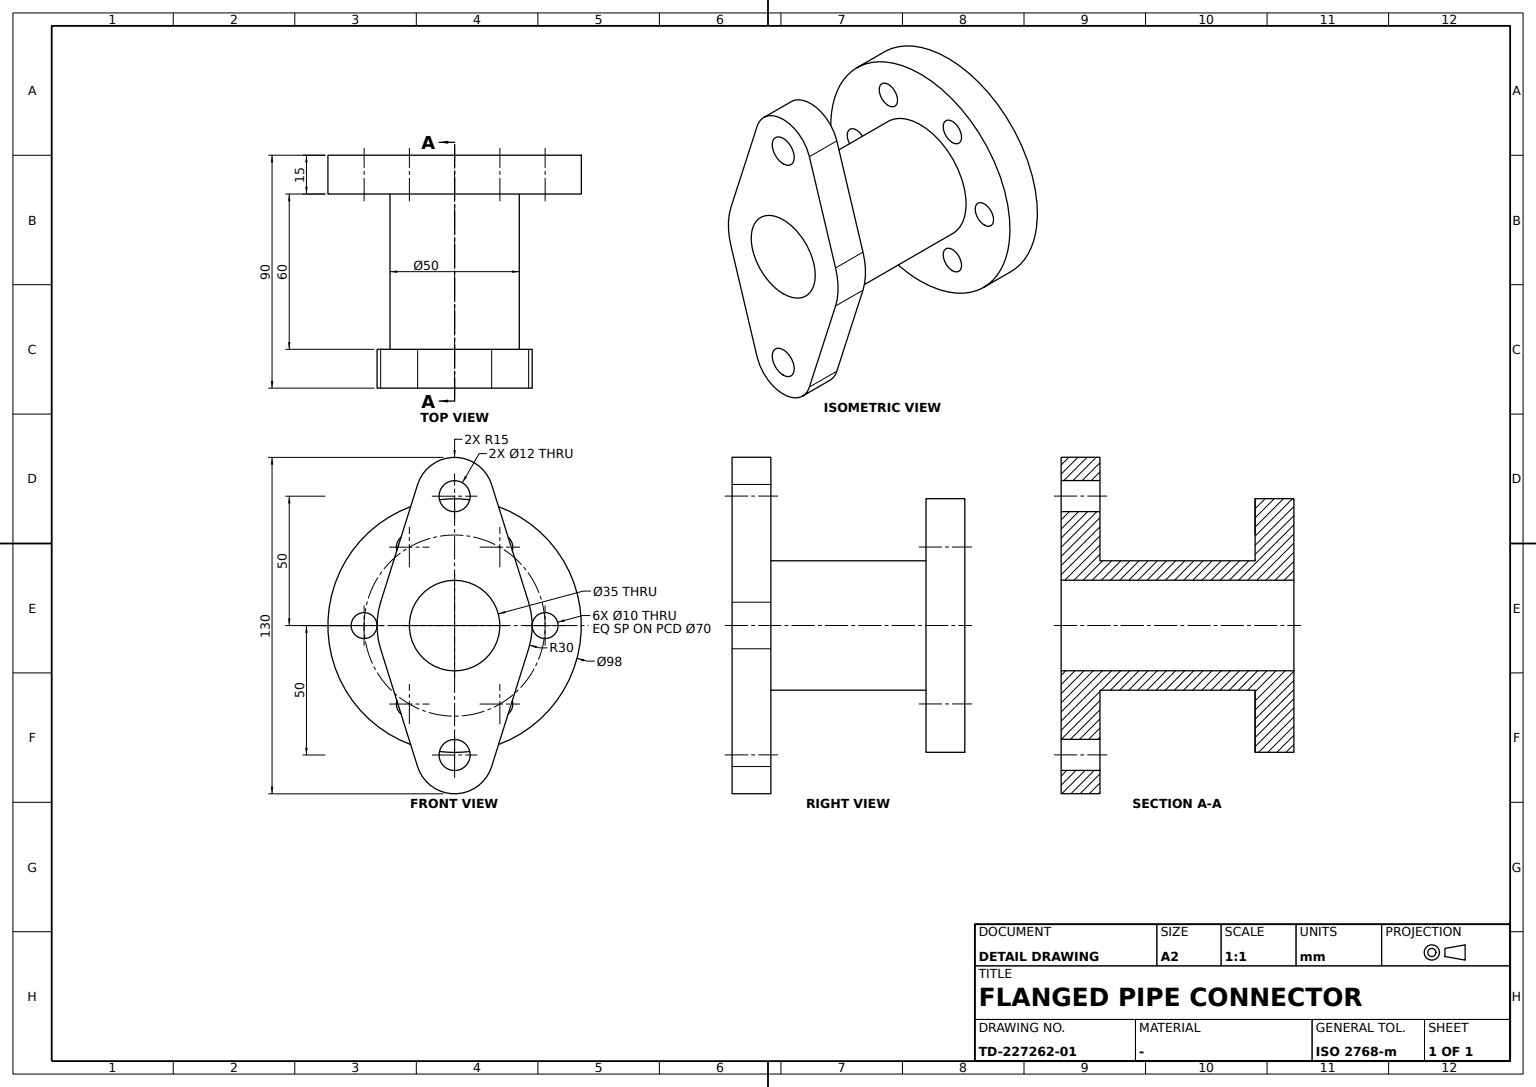
CATIA V5 part; units mm, degrees
sketch "Sketch1" plane through (0, 0, 0) normal (1, 0, 0) x (0, 1, 0)
  circle A0 centre (0, 0) radius 49
  circle A1 centre (-17.5, 30.3109) radius 5
  circle A2 centre (17.5, 30.3109) radius 5
  circle A3 centre (-17.5, -30.3109) radius 5
  circle A4 centre (17.5, -30.3109) radius 5
  circle A5 centre (35, 0) radius 5
  circle A6 centre (-35, 0) radius 5
  dimension "radius A0" = 49
  dimension "radius A1" = 5
  dimension "radius A5" = 5
  constraint symmetry A1 A2 y-axis
  constraint symmetry A1 A3 x-axis
  constraint symmetry A2 A4 x-axis
  constraint symmetry A5 A6 y-axis
extrude "Pad1" add sketch "Sketch1" along normal blind 15
sketch "Sketch2" plane through (15, 0, 0) normal (1, 0, 0) x (0, 1, 0)
  circle A0 centre (0, 0) radius 25
  dimension "radius A0" = 25
extrude "Pad2" add sketch "Sketch2" along normal blind 60
sketch "Sketch3" plane through (75, 0, 0) normal (1, 0, 0) x (0, 1, 0)
  arc A0 (-28.6182, 9) -> (-28.6182, -9) centre (0, 0) ccw
  circle A1 centre (0, 50) radius 6
  arc A2 (14.3091, 54.5) -> (-14.3091, 54.5) centre (0, 50) ccw
  arc A3 (14.3091, -54.5) -> (-14.3091, -54.5) centre (0, -50) cw
  circle A4 centre (0, -50) radius 6
  line L0 (14.3091, 54.5) -> (28.6182, 9)
  line L1 (14.3091, -54.5) -> (28.6182, -9)
  point P0 (28.6182, -9)
  line L2 (-14.3091, -54.5) -> (-28.6182, -9)
  line L3 (-28.6182, 9) -> (-14.3091, 54.5)
  arc A5 (28.6182, -9) -> (28.6182, 9) centre (0, 0) ccw
  dimension "radius A0" = 30
  dimension "radius A1" = 6
  dimension "radius A2" = 15
  constraint symmetry A2 A3 x-axis
  constraint symmetry A1 A4 x-axis
  constraint tangency L0 A2
  constraint tangency L0 A0
  constraint tangency L1 A3
  constraint tangency L1 A0
  constraint tangency L2 A3
  constraint tangency L2 A0
  constraint tangency L3 A0
  constraint tangency L3 A2
  constraint coincidence A0 P0
  constraint coincidence A0 A5
extrude "Pad3" add sketch "Sketch3" along normal blind 15
sketch "Sketch4" plane through (90, 0, 0) normal (1, 0, 0) x (0, 1, 0)
  circle A0 centre (0, 0) radius 17.5
  dimension "radius A0" = 17.5
extrude "Pocket1" cut sketch "Sketch4" against normal through all
